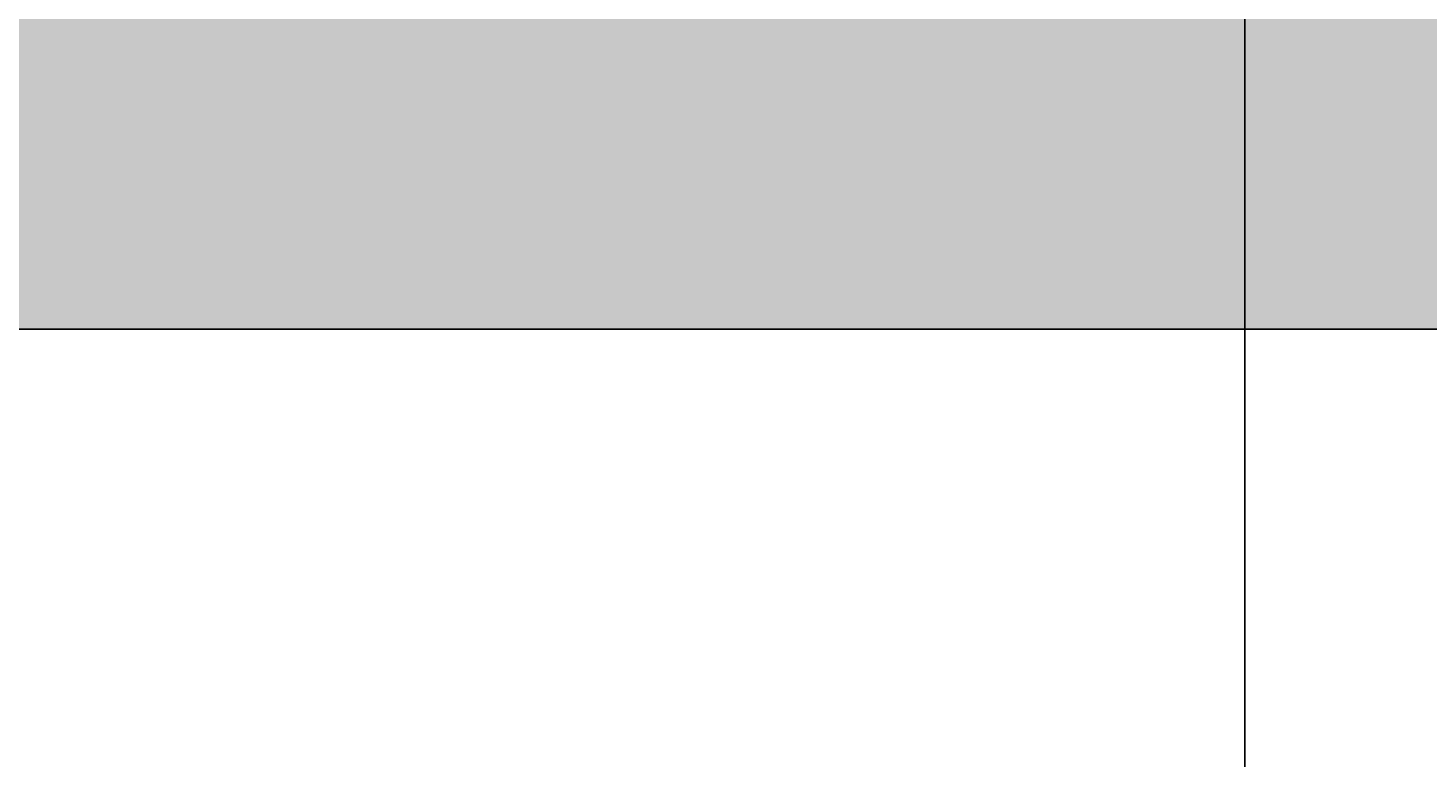
# Model space of a CAD drawing. Units: inches. Extents: x -301 to 715, y -607 to 364.
# Tile 12 of 141: x -19 to 18, y -493 to -474. Entities that reach past the tile are written whole.
import ezdxf

# ---------------------------------------------------------------- set-up
doc = ezdxf.new("R2010")
doc.units = ezdxf.units.IN
doc.header["$MEASUREMENT"] = 0
for name, color, linetype, lineweight in [('A-ANNO-DIMS', 2, 'Continuous', 18), ('A-GRND', 7, 'Continuous', 25), ('A-SECT-PATT', 8, 'Continuous', 13)]:
    doc.layers.add(name, color=color, linetype=linetype, lineweight=lineweight)
doc.styles.get("Standard").update_dxf_attribs({"font": 'arial.ttf'})
doc.dimstyles.get("Standard").update_dxf_attribs({"dimtxt": 0.18, "dimasz": 0.18, "dimexe": 0.18, "dimexo": 0.0625, "dimgap": 0.09, "dimtad": 0, "dimtih": 1, "dimtoh": 1, "dimdec": 1, "dimzin": 0, "dimdsep": 46, "dimlunit": 4, "dimtxsty": 'Standard', "dimcen": 0.09, "dimclrd": 3, "dimclre": 4, "dimclrt": 6, "dimadec": 0, "dimazin": 0, "dimtfac": 1, "dimtdec": 1, "dimtofl": 0, "dimtmove": 0, "dimatfit": 3, "dimfxl": 1, "dimtfill": 2, "dimtfillclr": 51, "dimtolj": 1, "dimtzin": 0, "dimarcsym": 0})

# ---------------------------------------------------------------- blocks, each defined once
blk = doc.blocks.new('*D176')
at = {"layer": 'A-ANNO-DIMS', "color": 4, "lineweight": -2, "transparency": 16777216}
for p, q in [((148.28, -324.477), (215.605, -324.477)), ((-15.22, -540.477), (215.605, -540.477))]:
    blk.add_line(p, q, dxfattribs=at)
at = {"layer": 'A-ANNO-DIMS', "color": 3, "lineweight": -2, "transparency": 16777216}
for p, q in [((215.425, -324.657), (215.425, -432.296)), ((215.425, -540.297), (215.425, -432.659))]:
    blk.add_line(p, q, dxfattribs=at)
at = {"layer": 'A-ANNO-DIMS', "color": 3, "transparency": 16777216}
for points in [[(215.395, -324.657), (215.455, -324.657), (215.425, -324.477)], [(215.395, -540.297), (215.455, -540.297), (215.425, -540.477)]]:
    blk.add_solid(points, dxfattribs=at)
at = {"layer": 'Defpoints', "color": 0, "transparency": 16777216}
for p in [(148.218, -324.477), (-15.282, -540.477), (215.425, -540.477)]:
    blk.add_point(p, dxfattribs=at)
at = {"layer": 'A-ANNO-DIMS', "color": 6, "transparency": 16777216, "insert": (215.425, -432.477), "char_height": 0.18, "attachment_point": 5, "bg_fill": 1, "box_fill_scale": 1.25, "bg_fill_color": 51, "bg_fill_transparency": 0}
blk.add_mtext('\\A1;18\'-0"', dxfattribs=at)
blk = doc.blocks.new('*D180')
at = {"layer": 'A-ANNO-DIMS', "color": 4, "lineweight": -2, "transparency": 16777216}
for p, q in [((-35.282, -463.54), (-35.282, -573.809)), ((12.718, -463.54), (12.718, -573.809))]:
    blk.add_line(p, q, dxfattribs=at)
at = {"layer": 'A-ANNO-DIMS', "color": 3, "lineweight": -2, "transparency": 16777216}
for p, q in [((-35.102, -573.629), (-11.615, -573.629)), ((12.538, -573.629), (-10.949, -573.629))]:
    blk.add_line(p, q, dxfattribs=at)
at = {"layer": 'A-ANNO-DIMS', "color": 3, "transparency": 16777216}
for points in [[(-35.102, -573.599), (-35.102, -573.659), (-35.282, -573.629)], [(12.538, -573.599), (12.538, -573.659), (12.718, -573.629)]]:
    blk.add_solid(points, dxfattribs=at)
at = {"layer": 'Defpoints', "color": 0, "transparency": 16777216}
for p in [(-35.282, -463.477), (12.718, -463.477), (12.718, -573.629)]:
    blk.add_point(p, dxfattribs=at)
at = {"layer": 'A-ANNO-DIMS', "color": 6, "transparency": 16777216, "insert": (-11.282, -573.629), "char_height": 0.18, "attachment_point": 5, "bg_fill": 1, "box_fill_scale": 1.25, "bg_fill_color": 51, "bg_fill_transparency": 0}
blk.add_mtext('\\A1;4\'-0"', dxfattribs=at)
blk = doc.blocks.new('*D181')
at = {"layer": 'A-ANNO-DIMS', "color": 4, "lineweight": -2, "transparency": 16777216}
for p, q in [((48.468, -433.54), (48.468, -573.809)), ((12.718, -463.54), (12.718, -573.809))]:
    blk.add_line(p, q, dxfattribs=at)
at = {"layer": 'A-ANNO-DIMS', "color": 3, "lineweight": -2, "transparency": 16777216}
for p, q in [((12.898, -573.629), (30.264, -573.629)), ((48.288, -573.629), (30.922, -573.629))]:
    blk.add_line(p, q, dxfattribs=at)
at = {"layer": 'A-ANNO-DIMS', "color": 3, "transparency": 16777216}
for points in [[(12.898, -573.599), (12.898, -573.659), (12.718, -573.629)], [(48.288, -573.599), (48.288, -573.659), (48.468, -573.629)]]:
    blk.add_solid(points, dxfattribs=at)
at = {"layer": 'Defpoints', "color": 0, "transparency": 16777216}
for p in [(48.468, -433.477), (12.718, -463.477), (48.468, -573.629)]:
    blk.add_point(p, dxfattribs=at)
at = {"layer": 'A-ANNO-DIMS', "color": 6, "transparency": 16777216, "insert": (30.593, -573.629), "char_height": 0.18, "attachment_point": 5, "bg_fill": 1, "box_fill_scale": 1.25, "bg_fill_color": 51, "bg_fill_transparency": 0}
blk.add_mtext('\\A1;3\'-0"', dxfattribs=at)
blk = doc.blocks.new('*D190')
at = {"layer": 'A-ANNO-DIMS', "color": 4, "lineweight": -2, "transparency": 16777216}
for p, q in [((129.193, -481.477), (-266.112, -481.477)), ((124.193, -511.477), (-266.112, -511.477))]:
    blk.add_line(p, q, dxfattribs=at)
at = {"layer": 'A-ANNO-DIMS', "color": 3, "lineweight": -2, "transparency": 16777216}
for p, q in [((-265.932, -481.657), (-265.932, -496.296)), ((-265.932, -511.297), (-265.932, -496.659))]:
    blk.add_line(p, q, dxfattribs=at)
at = {"layer": 'A-ANNO-DIMS', "color": 3, "transparency": 16777216}
for points in [[(-265.962, -481.657), (-265.902, -481.657), (-265.932, -481.477)], [(-265.962, -511.297), (-265.902, -511.297), (-265.932, -511.477)]]:
    blk.add_solid(points, dxfattribs=at)
at = {"layer": 'Defpoints', "color": 0, "transparency": 16777216}
for p in [(129.255, -481.477), (-265.932, -511.477), (124.255, -511.477)]:
    blk.add_point(p, dxfattribs=at)
at = {"layer": 'A-ANNO-DIMS', "color": 6, "transparency": 16777216, "insert": (-265.932, -496.477), "char_height": 0.18, "attachment_point": 5, "bg_fill": 1, "box_fill_scale": 1.25, "bg_fill_color": 51, "bg_fill_transparency": 0}
blk.add_mtext('\\A1;2\'-6"', dxfattribs=at)
blk = doc.blocks.new('*D191')
at = {"layer": 'A-ANNO-DIMS', "color": 4, "lineweight": -2, "transparency": 16777216}
for p, q in [((129.193, -481.477), (-266.112, -481.477)), ((114.193, -540.477), (-266.112, -540.477))]:
    blk.add_line(p, q, dxfattribs=at)
at = {"layer": 'A-ANNO-DIMS', "color": 3, "lineweight": -2, "transparency": 16777216}
for p, q in [((-265.932, -481.657), (-265.932, -510.797)), ((-265.932, -540.297), (-265.932, -511.158))]:
    blk.add_line(p, q, dxfattribs=at)
at = {"layer": 'A-ANNO-DIMS', "color": 3, "transparency": 16777216}
for points in [[(-265.962, -481.657), (-265.902, -481.657), (-265.932, -481.477)], [(-265.962, -540.297), (-265.902, -540.297), (-265.932, -540.477)]]:
    blk.add_solid(points, dxfattribs=at)
at = {"layer": 'Defpoints', "color": 0, "transparency": 16777216}
for p in [(129.255, -481.477), (-265.932, -540.477), (114.255, -540.477)]:
    blk.add_point(p, dxfattribs=at)
at = {"layer": 'A-ANNO-DIMS', "color": 6, "transparency": 16777216, "insert": (-265.932, -510.977), "char_height": 0.18, "attachment_point": 5, "bg_fill": 1, "box_fill_scale": 1.25, "bg_fill_color": 51, "bg_fill_transparency": 0}
blk.add_mtext('\\A1;4\'-11"', dxfattribs=at)

msp = doc.modelspace()

# ---------------------------------------------------------------- hatches: boundary and pattern name
at = {"layer": 'A-SECT-PATT'}
h = msp.add_hatch(dxfattribs=at)
h.set_pattern_fill('AR-CONC', color=256, scale=0.5)
h.set_pattern_definition([(50, (10.3213, 33.8764), (3.586301, -0.31376), [0.375, -4.125]), (355, (10.3213, 33.8764), (-0.693757, 3.76096), [0.3, -3.3]), (100.45144, (10.62, 33.8502), (2.892544, 3.4472), [0.3187, -3.50571]), (46.1842, (10.3213, 34.8764), (5.336207, -0.827596), [0.5625, -6.1875]), (96.6356, (10.766, 34.8074), (4.67331, 4.870593), [0.47805, -5.25857]), (351.1842, (10.321, 34.8764), (4.67331, 4.870593), [0.45, -4.95]), (21, (10.8213, 34.6264), (2.984535, -2.013094), [0.375, -4.125]), (326, (10.8213, 34.6264), (1.216577, 3.62575), [0.3, -3.3]), (71.45144, (11.07, 34.4586), (4.201112, 1.612656), [0.3187, -3.50571]), (37.5, (10.3213, 33.8764), (0.0607993, 1.6644693), [0, -3.26, 0, -3.35, 0, -3.3125]), (7.5, (10.3213, 33.8764), (1.3153477, 1.9720586), [0, -1.91, 0, -3.185, 0, -1.2625]), (327.5, (9.2063, 33.8764), (2.6691122, -0.1127744), [0, -1.25, 0, -3.9, 0, -5.175]), (317.5, (8.7063, 33.8764), (2.915931, 0.500525), [0, -1.625, 0, -2.59, 0, -3.675])])
h.paths.add_polyline_path([(-56.282, -535.477), (-61.282, -535.477), (-61.282, -540.477), (-15.282, -540.477), (-15.282, -535.477), (-20.282, -535.477)])
h.paths.add_polyline_path([(119.255, -535.477), (114.255, -535.477), (114.255, -540.477), (163.255, -540.477), (163.255, -535.477), (158.255, -535.477)])
h.paths.add_polyline_path([(-206.282, -471.477), (-209.282, -471.477), (-209.282, -481.477), (-206.282, -481.477), (-194.282, -481.477), (-194.282, -471.477)])
h.paths.add_polyline_path([(-41.282, -481.477), (-41.282, -471.477), (-185.282, -471.477), (-185.282, -481.477), (-180.282, -481.477)])
h.paths.add_polyline_path([(134.255, -481.477), (134.255, -471.477), (-35.282, -471.477), (-35.282, -481.477), (-30.282, -481.477)])
h.paths.add_polyline_path([(155.218, -481.477), (158.218, -481.477), (158.218, -471.477), (153.218, -471.477), (143.218, -471.477), (143.218, -481.477), (148.255, -481.477)])
h.paths.add_polyline_path([(-193.88, -356.477), (-193.904, -361.477), (143.218, -361.477), (143.218, -356.477)])

# ---------------------------------------------------------------- linework, layer by layer
at = {"layer": 'A-GRND'}
msp.add_line((-206.282, -481.477), (155.218, -481.477), dxfattribs=at)

# ---------------------------------------------------------------- dimensions: what is measured, and where the dimension line sits
at = {"layer": 'A-ANNO-DIMS'}
for base, p1, p2, picture, middle in [((215.425, -540.477), (148.218, -324.477), (-15.282, -540.477), '*D176', (215.425, -432.477)), ((-265.932, -540.477), (129.255, -481.477), (114.255, -540.477), '*D191', (-265.932, -510.977)), ((-265.932, -511.477), (129.255, -481.477), (124.255, -511.477), '*D190', (-265.932, -496.477))]:
    dim = msp.add_linear_dim(base=base, p1=p1, p2=p2, angle=90, dimstyle='Standard', override={"dimdec": 1, "dimlfac": 1, "dimrnd": 0, "dimzin": 1, "dimdsep": 46, "dimlunit": 4, "dimfrac": 2}, dxfattribs=at)
    dim.commit()
    dim.dimension.update_dxf_attribs({"geometry": picture, "text_midpoint": middle})
for base, p1, p2, picture, middle in [((48.467984, -573.628877), (12.717984, -463.47741), (48.467984, -433.47741), '*D181', (30.592984, -573.628877)), ((12.718, -573.629), (-35.282, -463.477), (12.718, -463.477), '*D180', (-11.282, -573.629))]:
    dim = msp.add_linear_dim(base=base, p1=p1, p2=p2, dimstyle='Standard', override={"dimdec": 1, "dimlfac": 1, "dimrnd": 0, "dimzin": 1, "dimdsep": 46, "dimlunit": 4, "dimfrac": 2}, dxfattribs=at)
    dim.commit()
    dim.dimension.update_dxf_attribs({"geometry": picture, "text_midpoint": middle})

doc.saveas('drawing.dxf')
